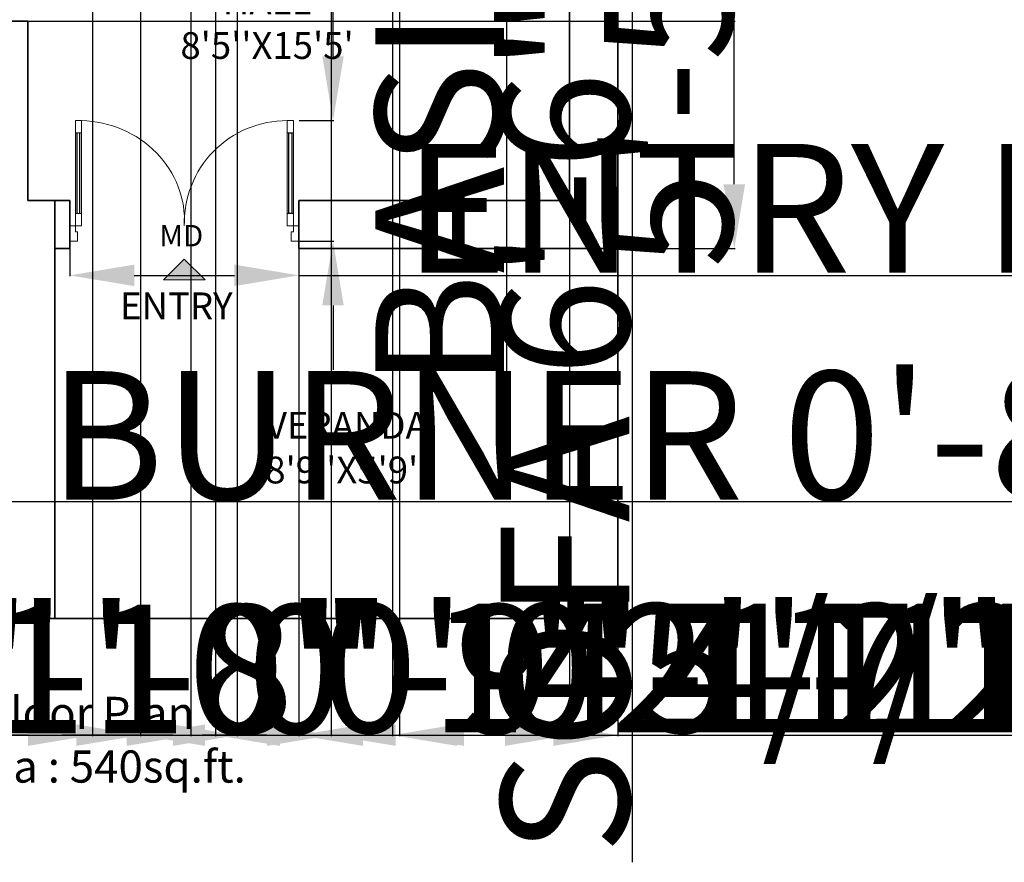
# Model space of a CAD drawing. Units: inches. Extents: x 2236 to 2927, y 1577 to 2452.
# Tile 2 of 9: x 2511 to 2695, y 1679 to 1836. Entities that reach past the tile are written whole.
import ezdxf

# ---------------------------------------------------------------- set-up
doc = ezdxf.new("R2010")
doc.units = ezdxf.units.IN
for name, color, linetype, lineweight in [('A-ANNO-DIMS', 2, 'Continuous', 18), ('A-ANNO-SYMB', 7, 'Continuous', 18), ('A-ANNO-TEXT', 7, 'Continuous', 18), ('A-AREA-IDEN', 7, 'Continuous', 18), ('Doors', 150, 'Continuous', 18), ('Wall', 7, 'Continuous', 35)]:
    doc.layers.add(name, color=color, linetype=linetype, lineweight=lineweight)
doc.layers.add('Glaz', color=92, linetype='Continuous')
doc.styles.get("Standard").update_dxf_attribs({"font": 'arial.ttf'})
doc.dimstyles.get("Standard").update_dxf_attribs({"dimtxt": 24, "dimasz": 12, "dimexe": 0.18, "dimexo": 0.0625, "dimgap": 0.09, "dimtad": 1, "dimdec": 1, "dimzin": 0, "dimdsep": 46, "dimlunit": 4, "dimtxsty": 'Standard', "dimcen": 0.09, "dimadec": 0, "dimazin": 0, "dimtfac": 1, "dimtdec": 1, "dimtofl": 0, "dimtmove": 0, "dimatfit": 3, "dimfxl": 1, "dimtolj": 1, "dimtzin": 0, "dimarcsym": 0})

# ---------------------------------------------------------------- blocks, each defined once
blk = doc.blocks.new('A$C13CE0A17')
at = {"layer": 'Doors'}
for p, q in [((0, 0.61), (0, 0.69)), ((0, 0.69), (0.04, 0.69)), ((0.04, 0.69), (0.04, 0.61)), ((0, 0.61), (0, 0.08)), ((0.04, 0.61), (0, 0.61)), ((0.04, 0.61), (0, 0.61)), ((0.03, 0.61), (0.01, 0.61)), ((0.04, 0.08), (0.04, 0.61)), ((0, 0.08), (0, 0)), ((0.04, 0.08), (0, 0.08)), ((0, 0.08), (0.04, 0.08)), ((0.01, 0.08), (0.03, 0.08)), ((0.04, 0), (0.04, 0.08)), ((-0.035, 0), (-0.035, -0.1)), ((0, 0), (-0.035, 0)), ((0, 0), (0.04, 0)), ((0, -0.04), (0, 0)), ((0.015, -0.04), (0, -0.04)), ((0.015, -0.05), (0.015, -0.04)), ((0.015, -0.1), (0.015, -0.05)), ((-0.035, -0.1), (0.015, -0.1))]:
    blk.add_line(p, q, dxfattribs=at)
for points in [[(1.39, 0.69), (1.39, 0.61), (1.43, 0.61), (1.43, 0.69)], [(1.39, 0.08), (1.39, 0.61), (1.43, 0.61), (1.43, 0.08)], [(1.39, 0), (1.39, 0.08), (1.43, 0.08), (1.43, 0)], [(1.43, 0), (1.465, 0), (1.465, -0.1), (1.415, -0.1), (1.415, -0.05), (1.415, -0.04), (1.43, -0.04)]]:
    blk.add_lwpolyline(points, close=True, dxfattribs=at)
blk.add_arc((1.3872, 0.017), 0.673, 89.76573, 181.44381, dxfattribs=at)
blk.add_ellipse((0.0389, 0.0511), major_axis=(0.6669, -0.1217), ratio=0.940794, start_param=0.11153, end_param=1.73917, dxfattribs=at)
at = {"layer": 'Glaz'}
for p, q in [((0.01, 0.61), (0.01, 0.08)), ((0.03, 0.08), (0.03, 0.61))]:
    blk.add_line(p, q, dxfattribs=at)
blk.add_lwpolyline([(1.4, 0.08), (1.4, 0.61), (1.42, 0.61), (1.42, 0.08)], close=True, dxfattribs=at)
blk = doc.blocks.new('DIRECTION-ARROWHEAD')
h = blk.add_hatch(color=256)
h.dxf.hatch_style = 1
h.paths.add_polyline_path([(3.87, 3.87), (0, 7.74), (0, 0)])
for p, q in [((0, 7.74), (0, 0)), ((3.87, 3.87), (0, 7.74)), ((3.87, 3.87), (0, 0))]:
    blk.add_line(p, q)
blk = doc.blocks.new('*D24')
at = {"layer": 'A-ANNO-DIMS', "color": 0, "lineweight": -2, "transparency": 16777216}
for p, q in [((2478.46, 1747), (2478.46, 1745.71)), ((2486.29, 1747), (2486.29, 1745.71)), ((2466.46, 1745.89), (2454.46, 1745.89)), ((2498.29, 1745.89), (2806.59, 1745.89))]:
    blk.add_line(p, q, dxfattribs=at)
at = {"layer": 'A-ANNO-DIMS', "color": 0, "transparency": 16777216}
for points in [[(2466.46, 1747.89), (2466.46, 1743.89), (2478.46, 1745.89)], [(2498.29, 1747.89), (2498.29, 1743.89), (2486.29, 1745.89)]]:
    blk.add_solid(points, dxfattribs=at)
at = {"layer": 'Defpoints', "color": 0, "transparency": 16777216}
for p in [(2478.46, 1747.06), (2486.29, 1747.06), (2486.29, 1745.89)]:
    blk.add_point(p, dxfattribs=at)
at = {"layer": 'A-ANNO-DIMS', "color": 0, "transparency": 16777216, "insert": (2658.44, 1758.23), "char_height": 24, "attachment_point": 5}
blk.add_mtext('\\A1;BURNER 0\'-8" TYP.', dxfattribs=at)
blk = doc.blocks.new('*D26')
at = {"layer": 'A-ANNO-DIMS', "color": 0, "lineweight": -2, "transparency": 16777216}
for p, q in [((2602.14, 1988.47), (2602.14, 2000.47)), ((2603.9, 1976.47), (2601.96, 1976.47)), ((2603.9, 1964.32), (2601.96, 1964.32)), ((2602.14, 1952.32), (2602.14, 1767.47))]:
    blk.add_line(p, q, dxfattribs=at)
at = {"layer": 'A-ANNO-DIMS', "color": 0, "transparency": 16777216}
for points in [[(2600.14, 1988.47), (2604.14, 1988.47), (2602.14, 1976.47)], [(2600.14, 1952.32), (2604.14, 1952.32), (2602.14, 1964.32)]]:
    blk.add_solid(points, dxfattribs=at)
at = {"layer": 'Defpoints', "color": 0, "transparency": 16777216}
for p in [(2603.96, 1976.47), (2602.14, 1964.32), (2603.96, 1964.32)]:
    blk.add_point(p, dxfattribs=at)
at = {"layer": 'A-ANNO-DIMS', "color": 0, "transparency": 16777216, "insert": (2589.64, 1853.9), "char_height": 24, "attachment_point": 5, "rotation": 90}
blk.add_mtext('\\A1;BASIN 1\'-0"', dxfattribs=at)
blk = doc.blocks.new('*D32')
at = {"layer": 'A-ANNO-DIMS', "color": 0, "lineweight": -2, "transparency": 16777216}
for p, q in [((2613.91, 1933.08), (2625.73, 1933.08)), ((2625.55, 1921.08), (2625.55, 1867.08)), ((2613.91, 1855.08), (2625.73, 1855.08)), ((2625.55, 1855.08), (2625.55, 1678.61))]:
    blk.add_line(p, q, dxfattribs=at)
at = {"layer": 'A-ANNO-DIMS', "color": 0, "transparency": 16777216}
for points in [[(2623.55, 1921.08), (2627.55, 1921.08), (2625.55, 1933.08)], [(2623.55, 1867.08), (2627.55, 1867.08), (2625.55, 1855.08)]]:
    blk.add_solid(points, dxfattribs=at)
at = {"layer": 'Defpoints', "color": 0, "transparency": 16777216}
for p in [(2613.85, 1933.08), (2613.85, 1855.08), (2625.55, 1855.08)]:
    blk.add_point(p, dxfattribs=at)
at = {"layer": 'A-ANNO-DIMS', "color": 0, "transparency": 16777216, "insert": (2613.04, 1760.84), "char_height": 24, "attachment_point": 5, "rotation": 90}
blk.add_mtext('\\A1;SOFA 6\'-6"', dxfattribs=at)
blk = doc.blocks.new('*D34')
at = {"layer": 'A-ANNO-DIMS', "color": 0, "lineweight": -2, "transparency": 16777216}
for p, q in [((2520.69, 1794.44), (2520.69, 1787.92)), ((2563.35, 1794.44), (2563.35, 1787.92)), ((2532.69, 1788.1), (2551.35, 1788.1)), ((2563.35, 1788.1), (2926.83, 1788.1))]:
    blk.add_line(p, q, dxfattribs=at)
at = {"layer": 'A-ANNO-DIMS', "color": 0, "transparency": 16777216}
for points in [[(2532.69, 1790.1), (2532.69, 1786.1), (2520.69, 1788.1)], [(2551.35, 1790.1), (2551.35, 1786.1), (2563.35, 1788.1)]]:
    blk.add_solid(points, dxfattribs=at)
at = {"layer": 'Defpoints', "color": 0, "transparency": 16777216}
for p in [(2520.69, 1794.5), (2563.35, 1794.5), (2563.35, 1788.1)]:
    blk.add_point(p, dxfattribs=at)
at = {"layer": 'A-ANNO-DIMS', "color": 0, "transparency": 16777216, "insert": (2751.09, 1800.62), "char_height": 24, "attachment_point": 5}
blk.add_mtext('\\A1;ENTRY DOOR 3\'-6 1/2"', dxfattribs=at)
blk = doc.blocks.new('*D35')
at = {"layer": 'A-ANNO-DIMS', "color": 0, "lineweight": -2, "transparency": 16777216}
for p, q in [((2569.75, 1828.98), (2569.75, 1977.27)), ((2563.41, 1816.98), (2569.93, 1816.98)), ((2563.41, 1794.5), (2569.93, 1794.5)), ((2569.75, 1782.5), (2569.75, 1770.5))]:
    blk.add_line(p, q, dxfattribs=at)
at = {"layer": 'A-ANNO-DIMS', "color": 0, "transparency": 16777216}
for points in [[(2567.75, 1828.98), (2571.75, 1828.98), (2569.75, 1816.98)], [(2567.75, 1782.5), (2571.75, 1782.5), (2569.75, 1794.5)]]:
    blk.add_solid(points, dxfattribs=at)
at = {"layer": 'Defpoints', "color": 0, "transparency": 16777216}
for p in [(2563.35, 1816.98), (2569.75, 1816.98), (2563.35, 1794.5)]:
    blk.add_point(p, dxfattribs=at)
at = {"layer": 'A-ANNO-DIMS', "color": 0, "transparency": 16777216, "insert": (2557.25, 1909.13), "char_height": 24, "attachment_point": 5, "rotation": 90}
blk.add_mtext('\\A1;1\'-10 1/2"', dxfattribs=at)
blk = doc.blocks.new('*D45')
at = {"layer": 'A-ANNO-DIMS', "color": 0, "lineweight": -2, "transparency": 16777216}
for p, q in [((2622.91, 1858.08), (2644.78, 1858.08)), ((2644.6, 1805.08), (2644.6, 1846.08)), ((2622.91, 1793.08), (2644.78, 1793.08))]:
    blk.add_line(p, q, dxfattribs=at)
at = {"layer": 'A-ANNO-DIMS', "color": 0, "transparency": 16777216}
for points in [[(2642.6, 1846.08), (2646.6, 1846.08), (2644.6, 1858.08)], [(2642.6, 1805.08), (2646.6, 1805.08), (2644.6, 1793.08)]]:
    blk.add_solid(points, dxfattribs=at)
at = {"layer": 'Defpoints', "color": 0, "transparency": 16777216}
for p in [(2622.85, 1858.08), (2644.6, 1858.08), (2622.85, 1793.08)]:
    blk.add_point(p, dxfattribs=at)
at = {"layer": 'A-ANNO-DIMS', "color": 0, "transparency": 16777216, "insert": (2632.3, 1825.58), "char_height": 24, "attachment_point": 5, "rotation": 90}
blk.add_mtext('\\A1;5\'-5"', dxfattribs=at)
blk = doc.blocks.new('*D46')
at = {"layer": 'A-ANNO-DIMS', "color": 0, "lineweight": -2, "transparency": 16777216}
for p, q in [((2415.85, 1873.01), (2415.85, 1702.15)), ((2533.86, 1873.01), (2533.86, 1702.15)), ((2427.85, 1702.33), (2521.86, 1702.33))]:
    blk.add_line(p, q, dxfattribs=at)
at = {"layer": 'A-ANNO-DIMS', "color": 0, "transparency": 16777216}
for points in [[(2427.85, 1704.33), (2427.85, 1700.33), (2415.85, 1702.33)], [(2521.86, 1704.33), (2521.86, 1700.33), (2533.86, 1702.33)]]:
    blk.add_solid(points, dxfattribs=at)
at = {"layer": 'Defpoints', "color": 0, "transparency": 16777216}
for p in [(2415.85, 1873.08), (2533.86, 1873.08), (2533.86, 1702.33)]:
    blk.add_point(p, dxfattribs=at)
at = {"layer": 'A-ANNO-DIMS', "color": 0, "transparency": 16777216, "insert": (2474.85, 1714.67), "char_height": 24, "attachment_point": 5}
blk.add_mtext('\\A1;9\'-10"', dxfattribs=at)
blk = doc.blocks.new('*D48')
at = {"layer": 'A-ANNO-DIMS', "color": 0, "lineweight": -2, "transparency": 16777216}
for p, q in [((2524.86, 1915.51), (2524.86, 1702.15)), ((2533.86, 1915.51), (2533.86, 1702.15)), ((2512.86, 1702.33), (2500.86, 1702.33)), ((2545.86, 1702.33), (2621.84, 1702.33))]:
    blk.add_line(p, q, dxfattribs=at)
at = {"layer": 'A-ANNO-DIMS', "color": 0, "transparency": 16777216}
for points in [[(2512.86, 1704.33), (2512.86, 1700.33), (2524.86, 1702.33)], [(2545.86, 1704.33), (2545.86, 1700.33), (2533.86, 1702.33)]]:
    blk.add_solid(points, dxfattribs=at)
at = {"layer": 'Defpoints', "color": 0, "transparency": 16777216}
for p in [(2524.86, 1915.58), (2533.86, 1915.58), (2533.86, 1702.33)]:
    blk.add_point(p, dxfattribs=at)
at = {"layer": 'A-ANNO-DIMS', "color": 0, "transparency": 16777216, "insert": (2589.85, 1714.67), "char_height": 24, "attachment_point": 5}
blk.add_mtext('\\A1;0\'-9"', dxfattribs=at)
blk = doc.blocks.new('*D50')
at = {"layer": 'A-ANNO-DIMS', "color": 0, "lineweight": -2, "transparency": 16777216}
for p, q in [((2563.35, 1793.01), (2563.35, 1702.15)), ((2622.85, 1793.01), (2622.85, 1702.15)), ((2575.35, 1702.33), (2610.85, 1702.33)), ((2622.85, 1702.33), (2774.36, 1702.33))]:
    blk.add_line(p, q, dxfattribs=at)
at = {"layer": 'A-ANNO-DIMS', "color": 0, "transparency": 16777216}
for points in [[(2575.35, 1704.33), (2575.35, 1700.33), (2563.35, 1702.33)], [(2610.85, 1704.33), (2610.85, 1700.33), (2622.85, 1702.33)]]:
    blk.add_solid(points, dxfattribs=at)
at = {"layer": 'Defpoints', "color": 0, "transparency": 16777216}
for p in [(2563.35, 1793.08), (2622.85, 1793.08), (2622.85, 1702.33)]:
    blk.add_point(p, dxfattribs=at)
at = {"layer": 'A-ANNO-DIMS', "color": 0, "transparency": 16777216, "insert": (2704.61, 1714.83), "char_height": 24, "attachment_point": 5}
blk.add_mtext('\\A1;4\'-11 1/2"', dxfattribs=at)
blk = doc.blocks.new('*D51')
at = {"layer": 'A-ANNO-DIMS', "color": 0, "lineweight": -2, "transparency": 16777216}
for p, q in [((2644.6, 1862.15), (2644.6, 1994.46)), ((2512.91, 1862.15), (2644.78, 1862.15)), ((2644.6, 1847.53), (2644.6, 1850.15)), ((2512.91, 1835.53), (2644.78, 1835.53))]:
    blk.add_line(p, q, dxfattribs=at)
at = {"layer": 'A-ANNO-DIMS', "color": 0, "transparency": 16777216}
for points in [[(2642.6, 1850.15), (2646.6, 1850.15), (2644.6, 1862.15)], [(2642.6, 1847.53), (2646.6, 1847.53), (2644.6, 1835.53)]]:
    blk.add_solid(points, dxfattribs=at)
at = {"layer": 'Defpoints', "color": 0, "transparency": 16777216}
for p in [(2512.85, 1862.15), (2644.6, 1862.15), (2512.85, 1835.53)]:
    blk.add_point(p, dxfattribs=at)
at = {"layer": 'A-ANNO-DIMS', "color": 0, "transparency": 16777216, "insert": (2632.1, 1934.31), "char_height": 24, "attachment_point": 5, "rotation": 90}
blk.add_mtext('\\A1;2\'-2 1/2"', dxfattribs=at)
blk = doc.blocks.new('*D54')
at = {"layer": 'A-ANNO-DIMS', "color": 0, "lineweight": -2, "transparency": 16777216}
for p, q in [((2543.24, 1954.99), (2543.24, 1702.15)), ((2547.85, 1955.01), (2547.85, 1702.15)), ((2531.24, 1702.33), (2519.24, 1702.33)), ((2559.85, 1702.33), (2691.75, 1702.33))]:
    blk.add_line(p, q, dxfattribs=at)
at = {"layer": 'A-ANNO-DIMS', "color": 0, "transparency": 16777216}
for points in [[(2531.24, 1704.33), (2531.24, 1700.33), (2543.24, 1702.33)], [(2559.85, 1704.33), (2559.85, 1700.33), (2547.85, 1702.33)]]:
    blk.add_solid(points, dxfattribs=at)
at = {"layer": 'Defpoints', "color": 0, "transparency": 16777216}
for p in [(2543.24, 1955.06), (2547.85, 1955.08), (2547.85, 1702.33)]:
    blk.add_point(p, dxfattribs=at)
at = {"layer": 'A-ANNO-DIMS', "color": 0, "transparency": 16777216, "insert": (2631.8, 1714.83), "char_height": 24, "attachment_point": 5}
blk.add_mtext('\\A1;0\'-4 1/2"', dxfattribs=at)
blk = doc.blocks.new('*D55')
at = {"layer": 'A-ANNO-DIMS', "color": 0, "lineweight": -2, "transparency": 16777216}
for p, q in [((2582.18, 1986.01), (2582.18, 1702.15)), ((2613.85, 1986.01), (2613.85, 1702.15)), ((2594.18, 1702.33), (2601.85, 1702.33)), ((2613.85, 1702.33), (2746.16, 1702.33))]:
    blk.add_line(p, q, dxfattribs=at)
at = {"layer": 'A-ANNO-DIMS', "color": 0, "transparency": 16777216}
for points in [[(2594.18, 1704.33), (2594.18, 1700.33), (2582.18, 1702.33)], [(2601.85, 1704.33), (2601.85, 1700.33), (2613.85, 1702.33)]]:
    blk.add_solid(points, dxfattribs=at)
at = {"layer": 'Defpoints', "color": 0, "transparency": 16777216}
for p in [(2582.18, 1986.08), (2613.85, 1986.08), (2613.85, 1702.33)]:
    blk.add_point(p, dxfattribs=at)
at = {"layer": 'A-ANNO-DIMS', "color": 0, "transparency": 16777216, "insert": (2686, 1714.83), "char_height": 24, "attachment_point": 5}
blk.add_mtext('\\A1;2\'-7 1/2"', dxfattribs=at)
blk = doc.blocks.new('*D56')
at = {"layer": 'A-ANNO-DIMS', "color": 0, "lineweight": -2, "transparency": 16777216}
for p, q in [((2551.88, 1874.28), (2551.88, 1702.15)), ((2569.42, 1874.28), (2569.42, 1702.15)), ((2539.88, 1702.33), (2527.88, 1702.33)), ((2581.42, 1702.33), (2711.06, 1702.33))]:
    blk.add_line(p, q, dxfattribs=at)
at = {"layer": 'A-ANNO-DIMS', "color": 0, "transparency": 16777216}
for points in [[(2539.88, 1704.33), (2539.88, 1700.33), (2551.88, 1702.33)], [(2581.42, 1704.33), (2581.42, 1700.33), (2569.42, 1702.33)]]:
    blk.add_solid(points, dxfattribs=at)
at = {"layer": 'Defpoints', "color": 0, "transparency": 16777216}
for p in [(2551.88, 1874.34), (2569.42, 1874.34), (2569.42, 1702.33)]:
    blk.add_point(p, dxfattribs=at)
at = {"layer": 'A-ANNO-DIMS', "color": 0, "transparency": 16777216, "insert": (2652.24, 1714.83), "char_height": 24, "attachment_point": 5}
blk.add_mtext('\\A1;1\'-5 1/2"', dxfattribs=at)
blk = doc.blocks.new('*D58')
at = {"layer": 'A-ANNO-DIMS', "color": 0, "lineweight": -2, "transparency": 16777216}
for p, q in [((2466.86, 1734.91), (2466.86, 1702.15)), ((2486.98, 1734.91), (2486.98, 1702.15)), ((2454.86, 1702.33), (2442.86, 1702.33)), ((2498.98, 1702.33), (2572.7, 1702.33))]:
    blk.add_line(p, q, dxfattribs=at)
at = {"layer": 'A-ANNO-DIMS', "color": 0, "transparency": 16777216}
for points in [[(2454.86, 1704.33), (2454.86, 1700.33), (2466.86, 1702.33)], [(2498.98, 1704.33), (2498.98, 1700.33), (2486.98, 1702.33)]]:
    blk.add_solid(points, dxfattribs=at)
at = {"layer": 'Defpoints', "color": 0, "transparency": 16777216}
for p in [(2466.86, 1734.97), (2486.98, 1734.97), (2486.98, 1702.33)]:
    blk.add_point(p, dxfattribs=at)
at = {"layer": 'A-ANNO-DIMS', "color": 0, "transparency": 16777216, "insert": (2541.84, 1714.67), "char_height": 24, "attachment_point": 5}
blk.add_mtext('\\A1;1\'-8"', dxfattribs=at)
blk = doc.blocks.new('*D59')
at = {"layer": 'A-ANNO-DIMS', "color": 0, "lineweight": -2, "transparency": 16777216}
for p, q in [((2466.86, 1734.91), (2466.86, 1702.15)), ((2444.85, 1733.17), (2444.85, 1702.15)), ((2432.85, 1702.33), (2420.85, 1702.33)), ((2478.86, 1702.33), (2571.23, 1702.33))]:
    blk.add_line(p, q, dxfattribs=at)
at = {"layer": 'A-ANNO-DIMS', "color": 0, "transparency": 16777216}
for points in [[(2432.85, 1704.33), (2432.85, 1700.33), (2444.85, 1702.33)], [(2478.86, 1704.33), (2478.86, 1700.33), (2466.86, 1702.33)]]:
    blk.add_solid(points, dxfattribs=at)
at = {"layer": 'Defpoints', "color": 0, "transparency": 16777216}
for p in [(2466.86, 1734.97), (2444.85, 1733.23), (2466.86, 1702.33)]:
    blk.add_point(p, dxfattribs=at)
at = {"layer": 'A-ANNO-DIMS', "color": 0, "transparency": 16777216, "insert": (2531.04, 1714.67), "char_height": 24, "attachment_point": 5}
blk.add_mtext('\\A1;1\'-10"', dxfattribs=at)
blk = doc.blocks.new('*D64')
at = {"layer": 'A-ANNO-DIMS', "color": 0, "lineweight": -2, "transparency": 16777216}
for p, q in [((2569.42, 1874.28), (2569.42, 1702.15)), ((2580.85, 1860.01), (2580.85, 1702.15)), ((2557.42, 1702.33), (2545.42, 1702.33)), ((2592.85, 1702.33), (2743.4, 1702.33))]:
    blk.add_line(p, q, dxfattribs=at)
at = {"layer": 'A-ANNO-DIMS', "color": 0, "transparency": 16777216}
for points in [[(2557.42, 1704.33), (2557.42, 1700.33), (2569.42, 1702.33)], [(2592.85, 1704.33), (2592.85, 1700.33), (2580.85, 1702.33)]]:
    blk.add_solid(points, dxfattribs=at)
at = {"layer": 'Defpoints', "color": 0, "transparency": 16777216}
for p in [(2569.42, 1874.34), (2580.85, 1860.08), (2580.85, 1702.33)]:
    blk.add_point(p, dxfattribs=at)
at = {"layer": 'A-ANNO-DIMS', "color": 0, "transparency": 16777216, "insert": (2674.12, 1714.83), "char_height": 24, "attachment_point": 5}
blk.add_mtext('\\A1;0\'-11 1/2"', dxfattribs=at)

msp = doc.modelspace()

# ---------------------------------------------------------------- linework, layer by layer
at = {"layer": 'Wall'}
for p, q in [((2622.85, 2084.08), (2622.85, 1724.08)), ((2613.85, 1986.08), (2613.85, 1802.08)), ((2508.85, 1835.53), (2512.85, 1835.53)), ((2512.85, 1835.53), (2512.85, 1802.08)), ((2512.85, 1802.08), (2520.69, 1802.08)), ((2517.85, 1802.08), (2517.85, 1724.08)), ((2520.69, 1802.08), (2520.69, 1793.08)), ((2563.35, 1802.08), (2563.35, 1793.08)), ((2563.35, 1802.08), (2613.85, 1802.08)), ((2517.85, 1793.08), (2520.69, 1793.08)), ((2563.35, 1793.08), (2622.85, 1793.08)), ((2406.85, 1724.08), (2622.85, 1724.08))]:
    msp.add_line(p, q, dxfattribs=at)

# ---------------------------------------------------------------- block references
at = {"layer": 'A-ANNO-SYMB', "rotation": 89.99999999998953}
msp.add_blockref('DIRECTION-ARROWHEAD', (2545.88, 1787.28), dxfattribs=at)
at = {"layer": 'Doors', "xscale": 28.43646753377714, "yscale": 28.43646753377714, "zscale": 28.43646753377714}
msp.add_blockref('A$C13CE0A17', (2521.69, 1797.34), dxfattribs=at)

# ---------------------------------------------------------------- texts
at = {"layer": 'A-ANNO-TEXT'}
for s, height, p in [('MD', 4, (2537.36, 1793.5)), ('ENTRY', 5, (2530.03, 1779.91))]:
    msp.add_text(s, height=height, dxfattribs=at).set_placement(p)
at = {"layer": 'A-ANNO-TEXT', "insert": (2428.34, 1709.48), "char_height": 6, "attachment_point": 1}
msp.add_mtext_dynamic_manual_height_columns('\\pxqc;Ground Floor Plan\\PBuilt Up Area : 540sq.ft.', width=161.5717, gutter_width=45.58, heights=[0], dxfattribs=at)
at = {"layer": 'A-AREA-IDEN', "char_height": 5, "attachment_point": 1}
for s, insert in [("\\pxqc;HALL\\P8'5''X15'5'", (2538.73, 1841.81)), ("\\pxqc;VERANDA\\P8'9''X5'9''", (2553.61, 1762.63))]:
    msp.add_mtext_dynamic_manual_height_columns(s, width=37.4353, gutter_width=12.5, heights=[0], dxfattribs=dict(at, insert=insert))

# ---------------------------------------------------------------- dimensions: what is measured, and where the dimension line sits
at = {"layer": 'A-ANNO-DIMS'}
for base, p1, p2, text, picture, middle in [((2602.1407, 1964.3191), (2603.9633, 1976.4697), (2603.9633, 1964.3191), 'BASIN <>', '*D26', (2589.6414, 1853.8962)), ((2625.55, 1855.08), (2613.85, 1933.08), (2613.85, 1855.08), 'SOFA <>', '*D32', (2613.04, 1760.84))]:
    dim = msp.add_linear_dim(base=base, p1=p1, p2=p2, angle=270, text=text, dimstyle='Standard', override={"dimdec": 1, "dimlfac": 1, "dimrnd": 0, "dimzin": 1, "dimdsep": 46, "dimlunit": 4, "dimfrac": 2}, dxfattribs=at)
    dim.commit()
    dim.dimension.update_dxf_attribs({"geometry": picture, "text_midpoint": middle})
for base, p1, p2, picture, middle in [((2644.6, 1862.15), (2512.85, 1835.53), (2512.85, 1862.15), '*D51', (2632.1, 1934.31)), ((2569.75, 1816.98), (2563.35, 1794.5), (2563.35, 1816.98), '*D35', (2557.25, 1909.13)), ((2644.6, 1858.08), (2622.85, 1793.08), (2622.85, 1858.08), '*D45', (2632.3, 1825.58))]:
    dim = msp.add_linear_dim(base=base, p1=p1, p2=p2, angle=90, dimstyle='Standard', override={"dimdec": 1, "dimlfac": 1, "dimrnd": 0, "dimzin": 1, "dimdsep": 46, "dimlunit": 4, "dimfrac": 2}, dxfattribs=at)
    dim.commit()
    dim.dimension.update_dxf_attribs({"geometry": picture, "text_midpoint": middle})
for base, p1, p2, picture, middle in [((2613.85, 1702.33), (2582.18, 1986.08), (2613.85, 1986.08), '*D55', (2686, 1714.83)), ((2547.85, 1702.33), (2543.24, 1955.06), (2547.85, 1955.08), '*D54', (2631.8, 1714.83)), ((2533.86, 1702.33), (2524.86, 1915.58), (2533.86, 1915.58), '*D48', (2589.85, 1714.67)), ((2569.42, 1702.33), (2551.88, 1874.34), (2569.42, 1874.34), '*D56', (2652.24, 1714.83)), ((2580.85, 1702.33), (2569.42, 1874.34), (2580.85, 1860.08), '*D64', (2674.12, 1714.83)), ((2533.86, 1702.33), (2415.85, 1873.08), (2533.86, 1873.08), '*D46', (2474.85, 1714.67)), ((2622.85, 1702.33), (2563.35, 1793.08), (2622.85, 1793.08), '*D50', (2704.61, 1714.83)), ((2466.86, 1702.33), (2444.85, 1733.23), (2466.86, 1734.97), '*D59', (2531.04, 1714.67)), ((2486.98, 1702.33), (2466.86, 1734.97), (2486.98, 1734.97), '*D58', (2541.84, 1714.67))]:
    dim = msp.add_linear_dim(base=base, p1=p1, p2=p2, dimstyle='Standard', override={"dimdec": 1, "dimlfac": 1, "dimrnd": 0, "dimzin": 1, "dimdsep": 46, "dimlunit": 4, "dimfrac": 2}, dxfattribs=at)
    dim.commit()
    dim.dimension.update_dxf_attribs({"geometry": picture, "text_midpoint": middle})
for base, p1, p2, text, picture, middle in [((2563.35, 1788.1), (2520.69, 1794.5), (2563.35, 1794.5), 'ENTRY DOOR <>', '*D34', (2751.09, 1800.62)), ((2486.29, 1745.89), (2478.46, 1747.06), (2486.29, 1747.06), 'BURNER <> TYP.', '*D24', (2658.44, 1758.23))]:
    dim = msp.add_linear_dim(base=base, p1=p1, p2=p2, text=text, dimstyle='Standard', override={"dimdec": 1, "dimlfac": 1, "dimrnd": 0, "dimzin": 1, "dimdsep": 46, "dimlunit": 4, "dimfrac": 2}, dxfattribs=at)
    dim.commit()
    dim.dimension.update_dxf_attribs({"geometry": picture, "text_midpoint": middle})

doc.saveas('drawing.dxf')
